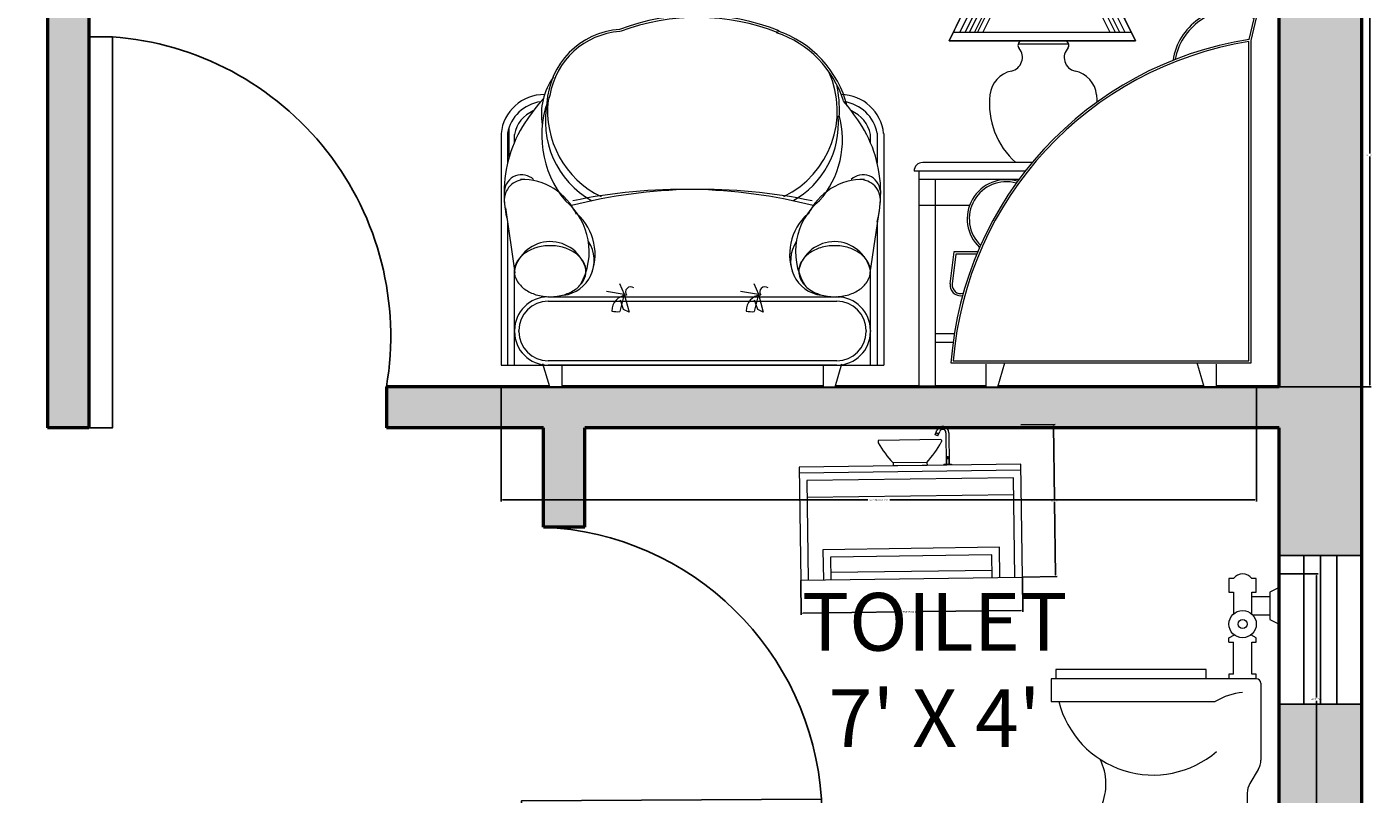
# Model space of a CAD drawing. Units: inches. Extents: x 1771 to 3025, y 319 to 889.
# Tile 6 of 35: x 1939 to 2102, y 620 to 713. Entities that reach past the tile are written whole.
import ezdxf

# ---------------------------------------------------------------- set-up
doc = ezdxf.new("R2010")
doc.units = ezdxf.units.IN
doc.header["$MEASUREMENT"] = 0
doc.set_wipeout_variables(frame=1)
for name, color, linetype, lineweight in [('A-ANNO-DIMS', 2, 'Continuous', 18), ('A-AREA-IDEN', 241, 'Continuous', 25), ('A-DOOR', 4, 'Continuous', 25), ('A-FLOR-FIXT', 8, 'Continuous', 18), ('A-FURN', 8, 'Continuous', 18), ('A-GLAZ', 40, 'Continuous', 25), ('A-WALL', 7, 'Continuous', 50), ('A-WALL-PATT', 254, 'Continuous', 13)]:
    doc.layers.add(name, color=color, linetype=linetype, lineweight=lineweight)
doc.styles.get("Standard").update_dxf_attribs({"font": 'arial.ttf'})
doc.dimstyles.get("Standard").update_dxf_attribs({"dimtxt": 0.18, "dimasz": 0.18, "dimexe": 0.18, "dimexo": 0.0625, "dimgap": 0.09, "dimtad": 0, "dimtih": 1, "dimtoh": 1, "dimdec": 4, "dimzin": 0, "dimdsep": 46, "dimtxsty": 'Standard', "dimcen": 0.09, "dimadec": 0, "dimazin": 0, "dimtfac": 1, "dimtdec": 4, "dimtofl": 0, "dimtmove": 0, "dimatfit": 3, "dimfxl": 1, "dimtolj": 1, "dimtzin": 0, "dimarcsym": 0})

# ---------------------------------------------------------------- blocks, each defined once
blk = doc.blocks.new('A$C425441F1')
for points in [[(1639.3, 0), (1667.3, 0), (1667.3, 55.3), (1748.6, 55.3), (1748.6, 807.4), (1761.1, 860.7), (1735.7, 880.7), (1703.4, 883.3), (1675.8, 879.6), (1656.2, 873.5), (1635.2, 863.3), (1619.6, 852.6), (1605.1, 839.5), (1596.7, 829.9), (1583.2, 810), (1573.2, 788.1), (1567.6, 767.7), (1566.5, 761.6), (1541.6, 750.9), (1510.7, 736.6), (1488.3, 725.3), (1464.5, 712.2), (1433.4, 693.6), (1409.1, 677.8), (1389.7, 664.2), (1388.2, 683.8), (1383.3, 700), (1376.2, 712), (1365.5, 723.2), (1352, 731.8), (1342.1, 735.4), (1331.7, 738.6), (1325, 742.7), (1317.7, 750.9), (1314.2, 758.8), (1312.9, 767.9), (1315.6, 780.8), (1321.1, 788.9), (1323.4, 793.7), (1323.6, 797.2), (1323.1, 800), (1320.5, 804.5), (1317.8, 806.7), (1317.8, 807.1), (1478.8, 807.1), (1345.8, 1080.7), (1177.3, 1080.7), (1044.3, 807.1), (1211.1, 807.1), (1211.1, 806.7), (1207.8, 803.9), (1205.8, 800.4), (1205.1, 796.3), (1207.6, 788.9), (1211.4, 783.4), (1213.5, 778.7), (1215.3, 769.8), (1215.1, 763.9), (1214.1, 759), (1208.8, 748.5), (1201.9, 741.7), (1195.3, 738), (1185.9, 735.4), (1176, 731.7), (1166.8, 726.4), (1159.9, 720.8), (1156.8, 717.7), (1149.3, 708.1), (1145.7, 701.6), (1143.6, 696.9), (1138.7, 669.7), (1138.7, 651.6), (1140.7, 631.8), (1142.6, 621.6), (1148.5, 600.5), (1162.8, 569), (1176.9, 547.8), (1188.6, 534.2), (1200, 523), (983, 523), (977.7, 522.3), (971.8, 519.6), (965.5, 512.8), (963.3, 506.8), (963, 503), (974.8, 503), (974.8, 3), (1013, 3), (1013, 103), (1053.6, 103), (1052.7, 96.1), (1051.6, 86.5), (1049.3, 63.6), (1048.6, 55.3), (1130.1, 55.3), (1130.1, 0), (1157.9, 0), (1174.1, 55.3), (1623.1, 55.6)], [(778.6, 0), (750.6, 0), (750.6, 50.4), (141.4, 50.4), (141.4, 0), (113.4, 0), (98.1, 50.4), (0, 50.4), (0, 590.4), (3.6, 609.1), (14.7, 633.7), (36.6, 658.7), (60.6, 673.3), (86.6, 680.5), (100.5, 681.5), (107.8, 698), (118.3, 717), (136.4, 751.3), (159.1, 779.5), (188.4, 803.6), (213.2, 817.4), (239.4, 827.1), (258.7, 831.4), (276, 833.4), (301.1, 842.1), (332.2, 850.9), (368.4, 858.6), (403.3, 863.5), (432.7, 865.8), (472.6, 866.2), (499.3, 864.8), (525, 862.1), (551.9, 857.9), (572.9, 853.6), (591.1, 849.1), (612.6, 842.8), (648, 830.4), (661.5, 823.7), (679.5, 815.2), (707.5, 798.2), (726.7, 783.3), (755.4, 754.4), (773.7, 729.8), (788.1, 704.9), (796.6, 686.1), (798.5, 681.2), (818, 677.9), (833.5, 672.3), (851.7, 661.6), (864.4, 650.3), (878.3, 632.1), (887.5, 611.7), (891.4, 595.2), (892, 590.4), (892, 50.4), (793.9, 50.4)]]:
    blk.add_wipeout(points)
for p, q in [((1044.3, 807.1), (1177.3, 1080.7)), ((1177.3, 1080.7), (1044.3, 807.1)), ((1188.8, 1068), (1069.3, 827.4)), ((1201.1, 1068), (1081.6, 827.4)), ((1211.2, 1068), (1091.7, 827.4)), ((1223.5, 1068), (1104, 827.4)), ((1230.5, 1068), (1110.9, 827.4)), ((1242.8, 1068), (1123.2, 827.4)), ((1171, 1067.8), (1351.9, 1067.8)), ((1177.3, 1080.7), (1345.8, 1080.7)), ((1345.8, 1080.7), (1177.3, 1080.7)), ((1299.6, 1068), (1419.2, 827.4)), ((1311.9, 1068), (1431.5, 827.4)), ((1322, 1068), (1441.5, 827.4)), ((1334.3, 1068), (1453.8, 827.4)), ((1345.8, 1080.7), (1478.8, 807.1)), ((1478.8, 807.1), (1345.8, 1080.7)), ((1735.7, 880.7), (1761.1, 860.7)), ((1733.6, 876.1), (1755.5, 858.7)), ((1744.1, 810.1), (1755.5, 858.7)), ((1748.6, 807.4), (1761.1, 860.7)), ((1053.8, 826.7), (1469.3, 826.7)), ((1478.8, 807.1), (1044.3, 807.1)), ((1044.3, 807.1), (1478.8, 807.1)), ((1205.6, 800), (1323.1, 800)), ((1211, 806.7), (1317.8, 806.7)), ((1743.6, 60.3), (1743.6, 805)), ((1748.6, 55.3), (1748.6, 807.4)), ((18.2, 603.6), (18.2, 536.8)), ((0, 590.4), (0, 50.4)), ((15, 591.1), (15, 521.6)), ((31, 569.9), (31, 588.4)), ((861, 569.9), (861, 588.4)), ((877, 591.1), (877, 521.6)), ((892, 590.4), (892, 50.4)), ((1222, 503), (963, 503)), ((974.8, 3), (974.8, 503)), ((1238.2, 523), (983, 523)), ((1206.8, 483), (974.8, 483)), ((1013, 3), (1013, 483)), ((10, 417.4), (32, 265.4)), ((882, 417.4), (860, 265.4)), ((1092.2, 423), (974.8, 423)), ((15, 385.1), (15, 50.4)), ((877, 385.1), (877, 50.4)), ((1055.6, 314.3), (1046.6, 240.3)), ((1111.1, 314.3), (1055.6, 314.3)), ((1060.1, 309.3), (1051.6, 239.7)), ((1109, 309.3), (1060.1, 309.3)), ((31, 50.4), (31, 272.3)), ((861, 50.4), (861, 272.3)), ((245.5, 223.1), (286.9, 216)), ((276.3, 240.8), (286.9, 216)), ((558.4, 223.2), (599.9, 216.1)), ((589.2, 240.9), (599.9, 216.1)), ((108.8, 209.4), (790.1, 209.4)), ((109.6, 209.4), (783, 209.4)), ((109.6, 199.4), (783, 199.4)), ((286.9, 216), (276.9, 175.2)), ((285.7, 179.9), (278.3, 201.7)), ((286.9, 216), (298.3, 173.5)), ((599.9, 216.1), (589.8, 175.3)), ((598.7, 180), (591.2, 201.8)), ((599.9, 216.1), (611.2, 173.6)), ((298.3, 173.5), (285.7, 179.9)), ((611.2, 173.6), (598.7, 180)), ((31.6, 128.4), (31.6, 131.4)), ((41.6, 128.4), (41.6, 131.4)), ((851, 131.4), (851, 128.4)), ((861, 131.4), (861, 128.4)), ((1056.5, 123), (1013, 123)), ((1053.6, 103), (1013, 103)), ((0, 50.4), (892, 50.4)), ((113.4, 0), (97.2, 53.4)), ((783, 60.4), (109.6, 60.4)), ((783, 50.4), (109.6, 50.4)), ((141.4, 50.4), (141.4, 0)), ((750.6, 50.4), (750.6, 0)), ((778.6, 0), (794.8, 53.4)), ((1048.6, 55.3), (1748.6, 55.3)), ((1054, 60.3), (1743.6, 60.3)), ((1129.9, 52.6), (1129.9, 0)), ((1157.9, 0), (1174.2, 55.6)), ((1639.3, 0), (1623.1, 55.6)), ((1667.3, 52.6), (1667.3, 0)), ((141.4, 0), (113.4, 0)), ((750.6, 0), (778.6, 0)), ((1129.9, 0), (1157.9, 0)), ((1667.3, 0), (1639.3, 0))]:
    blk.add_line(p, q)
for centre, radius, start, end in [((1708.4, 739.8), 143.6, 79.0486, 171.2543), ((458.1, 348.7), 517.8, 68.4843, 110.5916), ((458.1, 348.7), 512.8, 68.4843, 110.5916), ((1708.4, 739.8), 138.6, 79.5487, 170.0411), ((289.3, 651.4), 182.6, 93.9855, 176.965), ((289.3, 651.4), 177.6, 93.9855, 170.8791), ((563, 591.9), 246.9, 17.5917, 71.2419), ((563, 591.9), 251.9, 14.3659, 71.2419), ((1873.1, -6.5), 826.8, 98.9741, 175.711), ((1873.1, -6.5), 821.8, 99.0642, 175.3352), ((1183, 767.9), 32.3, 282.2329, 40.4775), ((1217.2, 796.3), 12.1, 120.8914, 217.6223), ((1345.2, 767.9), 32.3, 135.1029, 257.7671), ((1311.5, 796.3), 12.1, 322.3777, 59.1086), ((242.1, 635.9), 148, 144.2704, 189.5276), ((560.7, 643.7), 223.1, 296.1387, 23.9967), ((1203.5, 673.6), 64.2, 102.2329, 173.5671), ((1324.7, 673.6), 64.2, 6.4329, 77.7671), ((512.5, 645.7), 276.4, 357.4515, 12.4082), ((100.5, 580.5), 100.9, 89.5113, 174.4069), ((104.5, 574.5), 91, 97.7735, 169.4907), ((508.9, 316.7), 542.9, 139.0716, 146.5815), ((333.5, 586), 238.7, 156.9166, 219.7497), ((316.8, 619.2), 213.4, 167.2983, 240.5749), ((331.3, 643.7), 223.1, 173.6107, 243.8613), ((791.5, 580.5), 100.9, 5.5931, 89.1441), ((383.1, 316.7), 542.9, 33.4185, 40.1113), ((787.5, 574.5), 91, 10.5093, 82.2265), ((1322.1, 660.2), 183.7, 173.5671, 228.321), ((1206.1, 660.2), 183.7, 1.2452, 6.4329), ((104.5, 574.5), 74.8, 113.0142, 169.2704), ((579.4, 614.6), 207.2, 299.0365, 4.5654), ((578.1, 577), 217.9, 318.7723, 15.0106), ((787.5, 574.5), 74.8, 10.7296, 66.9858), ((301.8, 453.4), 294.8, 146.5815, 180), ((590.2, 453.4), 294.8, 0, 33.4185), ((983, 503), 20, 90, 180), ((56.7, 434.2), 49.4, 95.5103, 189.1585), ((48.3, 453.8), 40.5, 46.9039, 174.9451), ((49, 344.1), 139.3, 24.2628, 91.6479), ((843, 344.1), 139.3, 88.3521, 155.7372), ((843.7, 453.8), 40.5, 5.0549, 133.0961), ((835.3, 434.2), 49.4, 350.8415, 84.4897), ((1177.9, 391.7), 91.3, 73.3794, 227.0029), ((1177.9, 391.7), 86.3, 74.5383, 225.8439), ((301.8, 453.4), 294.8, 180, 193.379), ((468.1, -775.2), 1235.6, 77.9993, 104.2473), ((423.9, -775.2), 1235.6, 75.7527, 102.0007), ((590.2, 453.4), 294.8, 346.621, 0), ((52.4, 315.2), 153.2, 329.9033, 50.4478), ((839.6, 315.2), 153.2, 129.5522, 210.0967), ((92.5, 308.8), 126.8, 335.5815, 48.2351), ((799.5, 308.8), 126.8, 131.7649, 204.4185), ((114.7, 252.6), 85.8, 14.0074, 167.3648), ((106.2, 240.2), 87.4, 106.4444, 125.4727), ((114.5, 212.1), 116.8, 90, 106.4444), ((114.5, 212.1), 116.8, 73.5556, 90), ((135.5, 294.2), 81.5, 277.3995, 32.8179), ((122.8, 240.2), 87.4, 54.5273, 73.5556), ((756.5, 294.2), 81.5, 147.1821, 262.6005), ((777.3, 252.6), 85.8, 12.6352, 165.9926), ((769.2, 240.2), 87.4, 106.4444, 125.4727), ((777.5, 212.1), 116.8, 90, 106.4444), ((777.5, 212.1), 116.8, 73.5556, 90), ((785.8, 240.2), 87.4, 54.5273, 73.5556), ((74.1, 269.4), 43.1, 149.8309, 180), ((93.5, 258.1), 65.5, 125.4727, 149.8309), ((135.5, 258.1), 65.5, 30.1691, 54.5273), ((154.9, 269.4), 43.1, 0, 30.1691), ((737.1, 269.4), 43.1, 149.8309, 180), ((756.5, 258.1), 65.5, 125.4727, 149.8309), ((798.5, 258.1), 65.5, 30.1691, 54.5273), ((817.9, 269.4), 43.1, 0, 30.1691), ((74.1, 269.4), 43.1, 180, 210.1691), ((154.9, 269.4), 43.1, 329.8309, 0), ((737.1, 269.4), 43.1, 180, 210.1691), ((817.9, 269.4), 43.1, 329.8309, 0), ((93.5, 280.6), 65.5, 210.1691, 234.5273), ((106.2, 298.5), 87.4, 234.5273, 253.5556), ((122.8, 298.5), 87.4, 286.4444, 305.4727), ((135.5, 280.6), 65.5, 305.4727, 329.8309), ((302.4, 220.7), 12.2, 53.3958, 216.551), ((615.4, 220.8), 12.2, 53.3958, 216.551), ((756.5, 280.6), 65.5, 210.1691, 234.5273), ((769.2, 298.5), 87.4, 234.5273, 253.5556), ((785.8, 298.5), 87.4, 286.4444, 305.4727), ((798.5, 280.6), 65.5, 305.4727, 329.8309), ((1071.6, 237.3), 25.1, 173.0657, 279.7438), ((1071.6, 237.3), 20.1, 173.0657, 286.6808), ((109.6, 131.4), 78, 90, 180), ((109.6, 131.4), 68, 90, 180), ((114.5, 326.6), 116.8, 253.5556, 270), ((114.5, 326.6), 116.8, 270, 286.4444), ((294.4, 177.6), 35.9, 92.8846, 181.9), ((607.4, 177.7), 35.9, 92.8846, 181.9), ((777.5, 326.6), 116.8, 253.5556, 270), ((777.5, 326.6), 116.8, 270, 286.4444), ((783, 131.4), 78, 0, 90), ((783, 131.4), 68, 0, 90), ((271.5, 234.5), 59.6, 257.4358, 275.1883), ((584.4, 234.6), 59.6, 257.4358, 275.1883), ((109.6, 128.4), 78, 180, 270), ((109.6, 128.4), 68, 180, 270), ((783, 128.4), 68, 270, 0), ((783, 128.4), 78, 270, 0)]:
    blk.add_arc(centre, radius, start, end)
blk = doc.blocks.new('A$C062C426B')
for p, q in [((0.4867, 0.6739, -0.3429), (0.4867, 0.6365, -0.3429)), ((0.4992, 0.6739, -0.3429), (0.4867, 0.6739, -0.3429)), ((0.5616, 0.6739, -0.3429), (0.5491, 0.6739, -0.3429)), ((0.5616, 0.6365, -0.3429), (0.5616, 0.6739, -0.3429)), ((0.4867, 0.6365, -0.3429), (0.4992, 0.6365, -0.3429)), ((0.4992, 0.6365, -0.3429), (0.4992, 0.577, -0.3429)), ((0.5491, 0.6365, -0.3429), (0.5616, 0.6365, -0.3429)), ((0.5491, 0.577, -0.3429), (0.5491, 0.6365, -0.3429)), ((0.624, 0.649, -0.3429), (0.599, 0.6365, -0.3429)), ((0.599, 0.6365, -0.3429), (0.599, 0.5616, -0.3429)), ((0.624, 0.5491, -0.3429), (0.624, 0.649, -0.3429)), ((0.599, 0.624, -0.3429), (0.5491, 0.624, -0.3429)), ((0.5521, 0.5741, -0.3429), (0.599, 0.5741, -0.3429)), ((0.599, 0.5616, -0.3429), (0.624, 0.5491, -0.3429)), ((0.4867, 0.5117, -0.3429), (0.5017, 0.5192, -0.3429)), ((0.5616, 0.5117, -0.3429), (0.5466, 0.5192, -0.3429)), ((0.4867, 0.4992, -0.3429), (0.4867, 0.5117, -0.3429)), ((0.4867, 0.4992, -0.3429), (0.4992, 0.4992, -0.3429)), ((0.4992, 0.4118, -0.3429), (0.4992, 0.4992, -0.3429)), ((0.5491, 0.4118, -0.3429), (0.5491, 0.4992, -0.3429)), ((0.5491, 0.4992, -0.3429), (0.5616, 0.4992, -0.3429)), ((0.5616, 0.4992, -0.3429), (0.5616, 0.5117, -0.3429)), ((0.4243, 0.4243, -0.3429), (0.0125, 0.4243, -0.3429)), ((0.0125, 0.4243, -0.3429), (0.0125, 0.3994, -0.3429)), ((0.4243, 0.3994, -0.3429), (0.4243, 0.4243, -0.3429)), ((0.4992, 0.4118, -0.3429), (0.4867, 0.4118, -0.3429)), ((0.4867, 0.4118, -0.3429), (0.4867, 0.3994, -0.3429)), ((0.5616, 0.4118, -0.3429), (0.5491, 0.4118, -0.3429)), ((0.5616, 0.3994, -0.3429), (0.5616, 0.4118, -0.3429)), ((0.5616, 0.3994, -0.3429), (0, 0.3994, -0.3429)), ((0, 0.3994, -0.3429), (0, 0.337, -0.3429)), ((0.5741, 0.3869, -0.3429), (0.5741, 0.1761, -0.3429)), ((0, 0.337, -0.3429), (0.4493, 0.337, -0.3429)), ((0.567, 0.1504, -0.3429), (0.5438, 0.1117, -0.3429)), ((0.5366, 0.086, -0.3429), (0.5366, 0, -0.3429)), ((0.5366, 0.0374, -0.3429), (0.1248, 0.0374, -0.3429)), ((0.1248, 0.0374, -0.3429), (0.1248, 0, -0.3429)), ((0.5366, 0.0499, -0.3429), (0.1373, 0.0499, -0.3429)), ((0.1373, 0.0499, -0.3429), (0.1373, 0.0374, -0.3429))]:
    blk.add_line(p, q)
for radius in [0.0374, 0.0125]:
    blk.add_circle((0.5242, 0.5491, -0.3429), radius)
for centre, radius, start, end in [((0.5242, 0.6552, -0.3429), 0.0312, 36.8699, 143.1301), ((0.5616, 0.3869, -0.3429), 0.0125, 0, 90), ((0.2791, 0.4017, -0.3429), 0.2664, 194.0552, 310.7015), ((0.5429, 0.181, -0.3429), 0.1819, 95.9061, 120.9638), ((-0.0044, 0.1107, -0.3429), 0.1542, 336.7818, 25.8778), ((0.5242, 0.1761, -0.3429), 0.0499, 329.0362, 0), ((0.5866, 0.086, -0.3429), 0.0499, 149.0362, 180)]:
    blk.add_arc(centre, radius, start, end)
blk = doc.blocks.new('A$C127E6D2A')
for p, q in [((0.525, 0.915), (0.525, 0.9063)), ((0.525, 0.915), (0.525, 0.9063)), ((0.94, 0.92), (0.53, 0.92)), ((0.904, 0.9521), (0.9161, 0.9819)), ((0.9226, 0.9446), (0.904, 0.9521)), ((0.9275, 0.9563), (0.9088, 0.9639)), ((0.9282, 0.9582), (0.9095, 0.9657)), ((0.9226, 0.9446), (0.9346, 0.9744)), ((0.945, 0.915), (0.945, 0.9063)), ((0.975, 0.9647), (0.975, 0.756)), ((0.995, 0.964), (0.995, 0.756)), ((1.47, 0.75), (0, 0.75)), ((0, 0.75), (0, 0)), ((0.6225, 0.77), (0.6225, 0.75)), ((0.8475, 0.77), (0.6225, 0.77)), ((0.8475, 0.75), (0.6225, 0.75)), ((0.8475, 0.77), (0.8475, 0.75)), ((0.96, 0.756), (0.96, 0.75)), ((0.96, 0.756), (1.01, 0.756)), ((0.9925, 0.7905), (0.9775, 0.7905)), ((0.9775, 0.7905), (0.9775, 0.756)), ((0.982, 0.8022), (0.982, 0.7905)), ((0.988, 0.8022), (0.988, 0.7905)), ((0.9925, 0.7905), (0.9925, 0.756)), ((1.01, 0.756), (1.01, 0.75)), ((1.47, 0), (1.47, 0.75)), ((1.47, 0.71), (0, 0.71)), ((0.05, 0.66), (0.05, 0)), ((1.42, 0.66), (0.05, 0.66)), ((1.42, 0), (1.42, 0.66)), ((0.05, 0.55), (1.42, 0.55)), ((1.32, 0.2), (0.15, 0.2)), ((0.15, 0.2), (0.15, 0)), ((1.32, 0), (1.32, 0.2)), ((1.27, 0.15), (0.2, 0.15)), ((0.2, 0.15), (0.2, 0)), ((1.27, 0), (1.27, 0.15)), ((0.2, 0.05), (1.27, 0.05)), ((0, 0), (1.47, 0))]:
    blk.add_line(p, q)
blk.add_circle((0.985, 0.804), 0.0035)
for centre, radius, start, end in [((0.9541, 0.9665), 0.041, 356.58807, 157.98673), ((0.9541, 0.9665), 0.021, 355.23192, 157.98673), ((0.53, 0.915), 0.005, 90, 180), ((0.53, 0.9063), 0.005, 180, 209.45502), ((1.1676, 1.2664), 0.7372, 209.45502, 222.32259), ((0.3024, 1.2664), 0.7372, 317.67741, 330.54498), ((0.94, 0.915), 0.005, 0, 90), ((0.94, 0.9063), 0.005, 330.54498, 0)]:
    blk.add_arc(centre, radius, start, end)
blk = doc.blocks.new('DOOR-36B')
blk.add_lwpolyline([(0, 47.37), (2.84, 47.37), (2.84, 0), (0, 0)], close=True)
blk.add_arc((0.18, 11.12), 36.34, 350.3015, 85.8059)
blk = doc.blocks.new('DOOR-35')
blk.add_lwpolyline([(35.88, 36.19), (32.96, 36.3), (33.16, 0), (36, 0.05)], close=True)
blk.add_arc((35.23, 1.11), 35.26, 93.6879, 177.4925)
blk = doc.blocks.new('WIN-18')
for p, q in [((0, 0), (0, 10)), ((18, 0), (18, 10)), ((0, 7), (18, 7)), ((0, 5), (18, 5)), ((0, 3), (18, 3))]:
    blk.add_line(p, q)
blk = doc.blocks.new('*D38')
at = {"layer": 'A-ANNO-DIMS', "color": 0, "lineweight": -2, "transparency": 16777216}
for p, q in [((1996.59, 669.57), (1996.59, 655.74)), ((2087.99, 669.57), (2087.99, 655.74)), ((1996.77, 655.92), (2040.97, 655.92)), ((2087.81, 655.92), (2043.62, 655.92))]:
    blk.add_line(p, q, dxfattribs=at)
at = {"layer": 'A-ANNO-DIMS', "color": 0, "transparency": 16777216}
for points in [[(1996.77, 655.95), (1996.77, 655.89), (1996.59, 655.92)], [(2087.81, 655.95), (2087.81, 655.89), (2087.99, 655.92)]]:
    blk.add_solid(points, dxfattribs=at)
at = {"layer": 'Defpoints', "color": 0, "transparency": 16777216}
for p in [(1996.59, 669.63), (2087.99, 669.63), (2087.99, 655.92)]:
    blk.add_point(p, dxfattribs=at)
at = {"layer": 'A-ANNO-DIMS', "color": 0, "transparency": 16777216, "insert": (2042.29, 655.92), "char_height": 0.18, "attachment_point": 5}
blk.add_mtext('\\A1;ARMCHAIRS 91 TYP.', dxfattribs=at)
blk = doc.blocks.new('*D39')
at = {"layer": 'A-ANNO-DIMS', "color": 0, "lineweight": -2, "transparency": 16777216}
for p, q in [((2088.06, 725.72), (2101.88, 725.72)), ((2101.7, 725.54), (2101.7, 697.86)), ((2101.7, 669.81), (2101.7, 697.5)), ((2088.06, 669.63), (2101.88, 669.63))]:
    blk.add_line(p, q, dxfattribs=at)
at = {"layer": 'A-ANNO-DIMS', "color": 0, "transparency": 16777216}
for points in [[(2101.67, 725.54), (2101.73, 725.54), (2101.7, 725.72)], [(2101.67, 669.81), (2101.73, 669.81), (2101.7, 669.63)]]:
    blk.add_solid(points, dxfattribs=at)
at = {"layer": 'Defpoints', "color": 0, "transparency": 16777216}
for p in [(2087.99, 725.72), (2101.7, 725.72), (2087.99, 669.63)]:
    blk.add_point(p, dxfattribs=at)
at = {"layer": 'A-ANNO-DIMS', "color": 0, "transparency": 16777216, "insert": (2101.7, 697.68), "char_height": 0.18, "attachment_point": 5}
blk.add_mtext('\\A1;56 TYP.', dxfattribs=at)
blk = doc.blocks.new('*D52')
at = {"layer": 'A-ANNO-DIMS', "color": 0, "lineweight": -2, "transparency": 16777216}
for p, q in [((2090.79, 646.96), (2095.45, 646.96)), ((2095.27, 646.78), (2095.27, 631.98)), ((2095.27, 616.81), (2095.27, 631.61)), ((2090.79, 616.63), (2095.45, 616.63))]:
    blk.add_line(p, q, dxfattribs=at)
at = {"layer": 'A-ANNO-DIMS', "color": 0, "transparency": 16777216}
for points in [[(2095.24, 646.78), (2095.3, 646.78), (2095.27, 646.96)], [(2095.24, 616.81), (2095.3, 616.81), (2095.27, 616.63)]]:
    blk.add_solid(points, dxfattribs=at)
at = {"layer": 'Defpoints', "color": 0, "transparency": 16777216}
for p in [(2090.72, 646.96), (2095.27, 646.96), (2090.72, 616.63)]:
    blk.add_point(p, dxfattribs=at)
at = {"layer": 'A-ANNO-DIMS', "color": 0, "transparency": 16777216, "insert": (2095.27, 631.8), "char_height": 0.18, "attachment_point": 5}
blk.add_mtext('\\A1;WC 30 TYP.', dxfattribs=at)
blk = doc.blocks.new('*D54')
at = {"layer": 'A-ANNO-DIMS', "color": 0, "lineweight": -2, "transparency": 16777216}
for p, q in [((2032.85, 646.15), (2032.91, 642.01)), ((2059.67, 646.51), (2059.73, 642.37)), ((2033.09, 642.19), (2044.96, 642.35)), ((2059.54, 642.55), (2047.67, 642.39))]:
    blk.add_line(p, q, dxfattribs=at)
at = {"layer": 'A-ANNO-DIMS', "color": 0, "transparency": 16777216}
for points in [[(2033.09, 642.22), (2033.09, 642.16), (2032.91, 642.19)], [(2059.54, 642.58), (2059.54, 642.52), (2059.72, 642.55)]]:
    blk.add_solid(points, dxfattribs=at)
at = {"layer": 'Defpoints', "color": 0, "transparency": 16777216}
for p in [(2032.85, 646.21), (2059.67, 646.57), (2059.72, 642.55)]:
    blk.add_point(p, dxfattribs=at)
at = {"layer": 'A-ANNO-DIMS', "color": 0, "transparency": 16777216, "insert": (2046.31, 642.37), "char_height": 0.18, "attachment_point": 5}
blk.add_mtext('\\A1;WASH BASIN 27 TYP.', dxfattribs=at)
blk = doc.blocks.new('*D55')
at = {"layer": 'A-ANNO-DIMS', "color": 0, "lineweight": -2, "transparency": 16777216}
for p, q in [((2059.48, 665.02), (2063.62, 665.07)), ((2063.45, 664.89), (2063.57, 656.03)), ((2063.69, 646.81), (2063.57, 655.67)), ((2059.73, 646.57), (2063.87, 646.63))]:
    blk.add_line(p, q, dxfattribs=at)
at = {"layer": 'A-ANNO-DIMS', "color": 0, "transparency": 16777216}
for points in [[(2063.48, 664.89), (2063.42, 664.89), (2063.44, 665.07)], [(2063.72, 646.81), (2063.66, 646.81), (2063.69, 646.63)]]:
    blk.add_solid(points, dxfattribs=at)
at = {"layer": 'Defpoints', "color": 0, "transparency": 16777216}
for p in [(2059.42, 665.02), (2063.44, 665.07), (2059.67, 646.57)]:
    blk.add_point(p, dxfattribs=at)
at = {"layer": 'A-ANNO-DIMS', "color": 0, "transparency": 16777216, "insert": (2063.57, 655.85), "char_height": 0.18, "attachment_point": 5}
blk.add_mtext('\\A1;18 TYP.', dxfattribs=at)

msp = doc.modelspace()

# ---------------------------------------------------------------- hatches: boundary and pattern name
at = {"layer": 'A-WALL-PATT'}
h = msp.add_hatch(color=256, dxfattribs=at)
h.dxf.hatch_style = 1
h.paths.add_polyline_path([(1870.72, 888.63), (1799.72, 888.63), (1799.72, 878.63), (1870.72, 878.63)])
h.paths.add_polyline_path([(1968.77, 888.63), (1918.72, 888.63), (1918.72, 878.63), (1941.72, 878.63), (1941.72, 830.63), (1946.72, 830.63), (1946.72, 878.63), (1968.77, 878.63)])
h.paths.add_polyline_path([(2059.68, 888.63), (2016.77, 888.63), (2016.77, 878.63), (2037.72, 878.63), (2037.72, 794.63), (1941.72, 794.63), (1941.72, 758.63), (1941.72, 664.63), (1946.72, 664.63), (1946.72, 712), (1946.72, 789.63), (2054.72, 789.63), (2054.72, 794.63), (2042.33, 794.63), (2042.33, 798.62), (2042.33, 835.5), (2042.72, 878.63), (2059.68, 878.63)])
h.paths.add_polyline_path([(2100.72, 888.63), (2077.68, 888.63), (2077.68, 878.63), (2090.72, 878.63), (2090.72, 789.63), (2090.72, 768.61), (2100.72, 768.61)])
h.paths.add_polyline_path([(2100.72, 720.61), (2090.72, 720.61), (2090.72, 669.63), (1982.72, 669.63), (1982.72, 664.63), (2001.72, 664.63), (2001.72, 652.63), (2006.72, 652.63), (2006.72, 664.63), (2049.52, 664.63, -0.385549), (2050.52, 664.63), (2090.72, 664.63), (2090.72, 649.17), (2100.72, 649.17)])
edge = h.paths.add_edge_path()
edge.add_line((2100.72, 631.17), (2090.72, 631.17))
edge.add_line((2090.72, 631.17), (2090.72, 616.63))
edge.add_line((2090.72, 616.63), (2001.72, 616.63))
edge.add_line((2001.72, 616.63), (1982.72, 616.63))
edge.add_line((1982.72, 616.63), (1982.72, 611.63))
edge.add_line((1982.72, 611.63), (2024.67, 611.63))
edge.add_spline(control_points=[(2024.67, 611.63), (2027.58, 612.87), (2030.01, 613.31), (2032.47, 613.72)], knot_values=[484.321569, 484.321569, 484.321569, 484.321569, 625.498764, 625.498764, 625.498764, 625.498764], degree=3, periodic=0)
edge.add_line((2032.47, 613.72), (2033.2, 613.72))
edge.add_spline(control_points=[(2033.2, 613.72), (2035.66, 613.31), (2039.46, 612.87), (2042.2, 611.63)], knot_values=[484.321569, 484.321569, 484.321569, 484.321569, 625.498764, 625.498764, 625.498764, 625.498764], degree=3, periodic=0)
edge.add_line((2042.2, 611.63), (2090.72, 611.63))
edge.add_line((2090.72, 611.63), (2090.72, 581.11))
edge.add_line((2090.72, 581.11), (2100.72, 581.11))
edge.add_line((2100.72, 581.11), (2100.72, 631.17))
h.paths.add_polyline_path([(2100.72, 533.11), (2090.72, 533.11), (2090.72, 479.63), (1946.72, 479.63), (1946.72, 616.63), (1936.72, 616.63), (1936.72, 543.63), (1845.72, 543.63), (1845.72, 533.63), (1936.72, 533.63), (1936.72, 469.63), (2090.72, 469.63), (2090.72, 452.76), (2100.72, 452.76)])
h.paths.add_polyline_path([(2100.72, 404.76), (2090.72, 404.76), (2090.72, 393.63), (1936.72, 393.63), (1936.72, 383.63), (2100.72, 383.63)])
h.paths.add_polyline_path([(1905.72, 758.63), (1835.47, 758.63), (1835.47, 758.63), (1813.44, 758.63), (1809.72, 758.63), (1809.72, 842.59, -0.008336), (1808.42, 842.63), (1799.72, 842.63), (1799.72, 690.58), (1809.72, 690.58), (1809.72, 753.63), (1905.72, 753.63)])
h.paths.add_polyline_path([(1809.72, 642.58), (1799.72, 642.58), (1799.72, 533.63), (1809.72, 533.63), (1809.72, 581)])

# ---------------------------------------------------------------- linework, layer by layer
at = {"layer": 'A-WALL'}
for p, q in [((2100.72, 383.63), (2100.72, 888.43)), ((1946.72, 789.63), (1946.72, 669.63)), ((2090.72, 669.63), (2090.72, 789.63)), ((1941.72, 758.63), (1941.72, 664.63)), ((1946.72, 669.63), (1946.72, 664.63)), ((2090.72, 669.63), (1982.72, 669.63)), ((1982.72, 669.63), (1982.72, 664.63)), ((1946.72, 664.63), (1941.72, 664.63)), ((2001.72, 664.63), (1982.72, 664.63)), ((2001.72, 652.63), (2001.72, 664.63)), ((2090.72, 664.63), (2006.72, 664.63)), ((2006.72, 652.63), (2006.72, 664.63)), ((2090.72, 616.63), (2090.72, 664.63)), ((2006.72, 652.63), (2001.72, 652.63))]:
    msp.add_line(p, q, dxfattribs=at)

# ---------------------------------------------------------------- block references
at = {"layer": 'A-DOOR'}
msp.add_blockref('DOOR-36B', (1946.72, 664.63), dxfattribs=at)
at = {"layer": 'A-DOOR', "rotation": 269.9999999999959}
msp.add_blockref('DOOR-35', (1999.06, 652.63), dxfattribs=at)
at = {"layer": 'A-FLOR-FIXT', "xscale": 18.24536006826809, "yscale": 18.24536006826809, "zscale": 18.24536006826809, "rotation": 0.7699301504024306}
msp.add_blockref('A$C127E6D2A', (2032.85, 646.21, 15.15), dxfattribs=at)
at = {"layer": 'A-FLOR-FIXT', "xscale": 44.17762020618112, "yscale": 44.17762020618112, "zscale": 44.17762020618112}
msp.add_blockref('A$C062C426B', (2063.16, 616.63, 15.15), dxfattribs=at)
at = {"layer": 'A-GLAZ', "rotation": 269.9999999999989}
msp.add_blockref('WIN-18', (2090.72, 649.17), dxfattribs=at)

# ---------------------------------------------------------------- texts
at = {"layer": 'A-AREA-IDEN', "insert": (2006.32, 644.66), "char_height": 7, "attachment_point": 1}
msp.add_mtext_dynamic_manual_height_columns("\\pxqc;TOILET \\P7' X 4'", width=85.4611, gutter_width=1, heights=[0], dxfattribs=at)

# ---------------------------------------------------------------- dimensions: what is measured, and where the dimension line sits
at = {"layer": 'A-ANNO-DIMS'}
for base, p1, p2, angle, text, picture, middle in [((2063.44, 665.07), (2059.67, 646.57), (2059.42, 665.02), 90.7699, '<> TYP.', '*D55', (2063.57, 655.85)), ((2095.27, 646.96), (2090.72, 616.63), (2090.72, 646.96), 90, 'WC <> TYP.', '*D52', (2095.27, 631.8)), ((2059.72, 642.55), (2032.85, 646.21), (2059.67, 646.57), 0.7699, 'WASH BASIN <> TYP.', '*D54', (2046.31, 642.37))]:
    dim = msp.add_linear_dim(base=base, p1=p1, p2=p2, angle=angle, text=text, dimstyle='Standard', override={"dimdec": 0, "dimrnd": 0, "dimzin": 0, "dimlunit": 2}, dxfattribs=at)
    dim.commit()
    dim.dimension.update_dxf_attribs({"geometry": picture, "text_midpoint": middle})

# ---------------------------------------------------------------- next in the draw order: block references
at = {"layer": 'A-FURN', "xscale": 0.0519011286993662, "yscale": 0.0519011286993662, "zscale": 0.0519011286993662}
msp.add_blockref('A$C425441F1', (1996.59, 669.63), dxfattribs=at)

# ---------------------------------------------------------------- next in the draw order: dimensions: what is measured, and where the dimension line sits
at = {"layer": 'A-ANNO-DIMS'}
dim = msp.add_linear_dim(base=(2101.7, 725.72), p1=(2087.99, 669.63), p2=(2087.99, 725.72), angle=90, text='<> TYP.', dimstyle='Standard', override={"dimdec": 0, "dimrnd": 0, "dimzin": 0, "dimlunit": 2}, dxfattribs=at)
dim.commit()
dim.dimension.update_dxf_attribs({"geometry": '*D39', "text_midpoint": (2101.7, 697.68)})
dim = msp.add_linear_dim(base=(2087.99, 655.92), p1=(1996.59, 669.63), p2=(2087.99, 669.63), text='ARMCHAIRS <> TYP.', dimstyle='Standard', override={"dimdec": 0, "dimrnd": 0, "dimzin": 0, "dimlunit": 2}, dxfattribs=at)
dim.commit()
dim.dimension.update_dxf_attribs({"geometry": '*D38', "text_midpoint": (2042.29, 655.92)})

doc.saveas('drawing.dxf')
